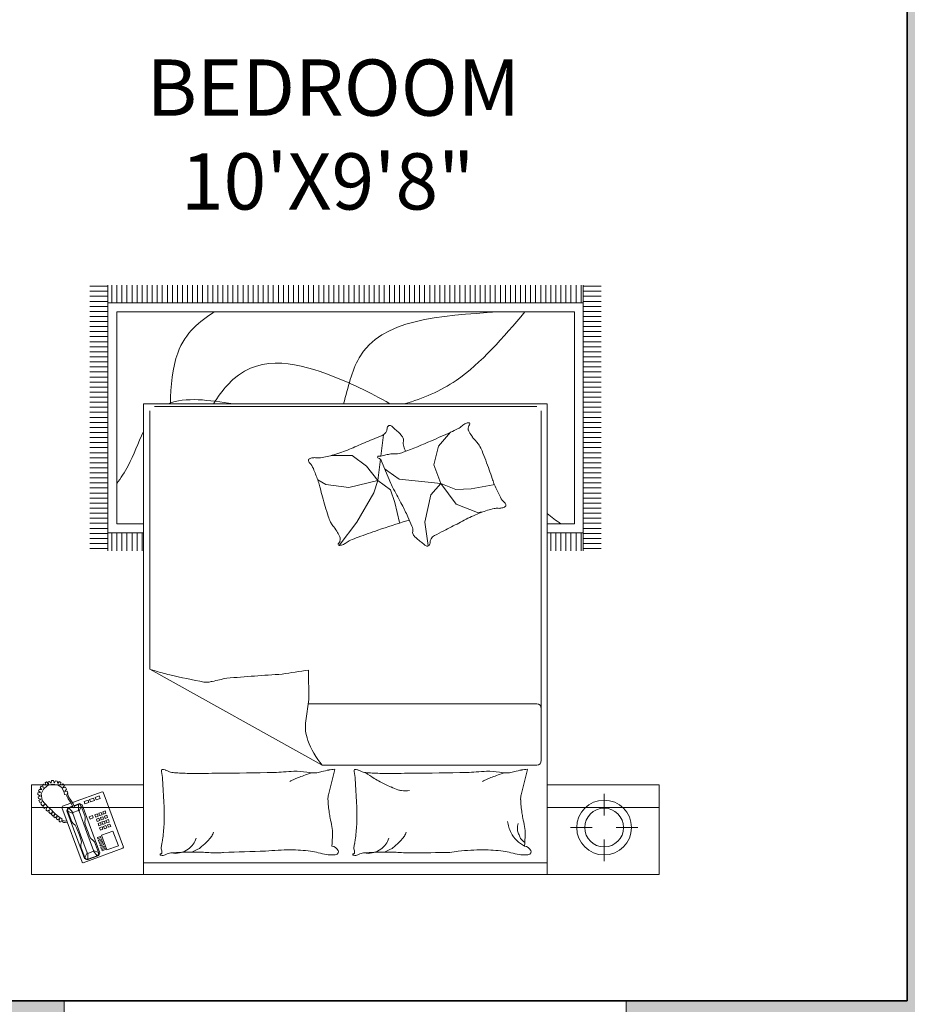
# Model space of a CAD drawing. Units: inches. Extents: x 311 to 815, y -527 to 136.
# Tile 4 of 21: x 445 to 539, y -474 to -368. Entities that reach past the tile are written whole.
import ezdxf

# ---------------------------------------------------------------- set-up
doc = ezdxf.new("R2010")
doc.units = ezdxf.units.IN
doc.header["$MEASUREMENT"] = 0
for name, color, linetype, lineweight in [('A-AREA-IDEN', 8, 'Continuous', 18), ('A-WALL-PATT', 242, 'Continuous', 13), ('wall', 1, 'Continuous', 35), ('win', 5, 'Continuous', 18)]:
    doc.layers.add(name, color=color, linetype=linetype, lineweight=lineweight)
doc.layers.add('furniture', color=50, linetype='Continuous', lineweight=13, transparency=0.8)
doc.styles.add('DIM_FONT', font='SIMPLEX.shx', dxfattribs={"width": 0.8})
doc.styles.get("Standard").update_dxf_attribs({"font": 'arial.ttf'})

# ---------------------------------------------------------------- blocks, each defined once
blk = doc.blocks.new('A$C4F634EDD')
for p, q in [((0, 2.6295), (0, 2.2295)), ((0.5, 2.6295), (0, 2.6295)), ((0.5, 2.6295), (2.3, 2.6295)), ((0.5, 0.5295), (0.5, 2.6295)), ((0.5, 2.2295), (0.5, 2.6295)), ((2.3, 2.6295), (2.3, 0.5295)), ((2.3, 2.6295), (2.8, 2.6295)), ((2.3, 2.2295), (2.3, 2.6295)), ((2.8, 2.6295), (2.8, 2.2295)), ((0.2457, 2.5697), (0.2457, 2.4733)), ((0.5, 2.5771), (2.3, 2.5771)), ((2.392, 2.5115), (2.5692, 2.5765)), ((2.4985, 2.5445), (2.5516, 2.564)), ((2.5062, 2.5454), (2.5487, 2.561)), ((2.5483, 2.5347), (2.5487, 2.561)), ((2.5487, 2.561), (2.5571, 2.56)), ((2.5615, 2.5536), (2.5514, 2.5318)), ((2.5516, 2.564), (2.5637, 2.5584)), ((2.5571, 2.56), (2.5615, 2.5536)), ((2.5615, 2.5536), (2.5791, 2.5058)), ((2.5637, 2.5584), (2.6418, 2.3458)), ((2.5692, 2.5765), (2.574, 2.5743)), ((2.574, 2.5743), (2.6638, 2.3298)), ((2.3898, 2.5066), (2.392, 2.5115)), ((2.4795, 2.2621), (2.3898, 2.5066)), ((2.412, 2.5007), (2.4634, 2.5196)), ((2.4634, 2.5196), (2.4875, 2.454)), ((2.4842, 2.5232), (2.47, 2.518)), ((2.47, 2.518), (2.472, 2.5127)), ((2.472, 2.5127), (2.4862, 2.5179)), ((2.4881, 2.5126), (2.4739, 2.5074)), ((2.4739, 2.5074), (2.4759, 2.502)), ((2.4759, 2.502), (2.4901, 2.5073)), ((2.4862, 2.5179), (2.4842, 2.5232)), ((2.4901, 2.5073), (2.4881, 2.5126)), ((2.4946, 2.5331), (2.4985, 2.5445)), ((2.5734, 2.3187), (2.4946, 2.5331)), ((2.5062, 2.5454), (2.5004, 2.5392)), ((2.5004, 2.5392), (2.5013, 2.5315)), ((2.5013, 2.5315), (2.5188, 2.4836)), ((2.5013, 2.5315), (2.5231, 2.5214)), ((2.5235, 2.5256), (2.5062, 2.5454)), ((2.5231, 2.5214), (2.5235, 2.5256)), ((2.5523, 2.4417), (2.5231, 2.5214)), ((2.5483, 2.5347), (2.5235, 2.5256)), ((2.5514, 2.5318), (2.5483, 2.5347)), ((2.5807, 2.4521), (2.5514, 2.5318)), ((2.5791, 2.5058), (2.5788, 2.4956)), ((2.4361, 2.4352), (2.412, 2.5007)), ((2.492, 2.5019), (2.4778, 2.4967)), ((2.4778, 2.4967), (2.4798, 2.4914)), ((2.4798, 2.4914), (2.494, 2.4966)), ((2.4959, 2.4913), (2.4817, 2.4861)), ((2.4817, 2.4861), (2.4837, 2.4808)), ((2.4837, 2.4808), (2.4979, 2.486)), ((2.4998, 2.4807), (2.4856, 2.4755)), ((2.4856, 2.4755), (2.4876, 2.4702)), ((2.4876, 2.4702), (2.5018, 2.4754)), ((2.5037, 2.47), (2.4895, 2.4648)), ((2.4895, 2.4648), (2.4915, 2.4595)), ((2.4915, 2.4595), (2.5057, 2.4647)), ((2.494, 2.4966), (2.492, 2.5019)), ((2.4979, 2.486), (2.4959, 2.4913)), ((2.5018, 2.4754), (2.4998, 2.4807)), ((2.5057, 2.4647), (2.5037, 2.47)), ((2.5188, 2.4836), (2.5256, 2.4761)), ((2.5256, 2.4761), (2.5342, 2.4692)), ((2.5342, 2.4692), (2.5405, 2.4574)), ((2.5788, 2.4956), (2.5767, 2.4848)), ((2.5767, 2.4848), (2.5795, 2.4717)), ((2.5795, 2.4717), (2.586, 2.454)), ((0.0957, 2.4197), (0.192, 2.4197)), ((0.2994, 2.4197), (0.3957, 2.4197)), ((2.4875, 2.454), (2.4361, 2.4352)), ((2.4457, 2.4146), (2.4563, 2.4185)), ((2.4563, 2.4185), (2.4602, 2.4078)), ((2.4634, 2.4211), (2.474, 2.425)), ((2.4673, 2.4104), (2.4634, 2.4211)), ((2.474, 2.425), (2.4779, 2.4143)), ((2.4811, 2.4276), (2.4917, 2.4315)), ((2.485, 2.4169), (2.4811, 2.4276)), ((2.4956, 2.4208), (2.485, 2.4169)), ((2.4917, 2.4315), (2.4956, 2.4208)), ((2.5405, 2.4574), (2.547, 2.4397)), ((2.5594, 2.4061), (2.547, 2.4397)), ((2.5523, 2.4417), (2.5875, 2.346)), ((2.5807, 2.4521), (2.6158, 2.3564)), ((2.5984, 2.4204), (2.586, 2.454)), ((2.6047, 2.4086), (2.5984, 2.4204)), ((2.4496, 2.4039), (2.4457, 2.4146)), ((2.4602, 2.4078), (2.4496, 2.4039)), ((2.4528, 2.3951), (2.4635, 2.399)), ((2.4567, 2.3844), (2.4528, 2.3951)), ((2.4674, 2.3883), (2.4567, 2.3844)), ((2.46, 2.3756), (2.4706, 2.3795)), ((2.4639, 2.365), (2.46, 2.3756)), ((2.4635, 2.399), (2.4674, 2.3883)), ((2.4779, 2.4143), (2.4673, 2.4104)), ((2.4706, 2.4016), (2.4812, 2.4055)), ((2.4745, 2.3909), (2.4706, 2.4016)), ((2.4706, 2.3795), (2.4745, 2.3689)), ((2.4851, 2.3949), (2.4745, 2.3909)), ((2.4777, 2.3821), (2.4883, 2.386)), ((2.4816, 2.3715), (2.4777, 2.3821)), ((2.4812, 2.4055), (2.4851, 2.3949)), ((2.4922, 2.3754), (2.4816, 2.3715)), ((2.4883, 2.4081), (2.4989, 2.412)), ((2.4922, 2.3975), (2.4883, 2.4081)), ((2.4883, 2.386), (2.4922, 2.3754)), ((2.5028, 2.4014), (2.4922, 2.3975)), ((2.4954, 2.3886), (2.5061, 2.3925)), ((2.4993, 2.378), (2.4954, 2.3886)), ((2.4989, 2.412), (2.5028, 2.4014)), ((2.51, 2.3819), (2.4993, 2.378)), ((2.5026, 2.3691), (2.5132, 2.373)), ((2.5061, 2.3925), (2.51, 2.3819)), ((2.5132, 2.373), (2.5171, 2.3624)), ((2.5238, 2.3769), (2.538, 2.3821)), ((2.5277, 2.3663), (2.5238, 2.3769)), ((2.5419, 2.3715), (2.5277, 2.3663)), ((2.538, 2.3821), (2.5419, 2.3715)), ((2.5622, 2.393), (2.5594, 2.4061)), ((2.5598, 2.372), (2.5601, 2.3822)), ((2.5774, 2.3242), (2.5598, 2.372)), ((2.5601, 2.3822), (2.5622, 2.393)), ((2.6133, 2.4017), (2.6047, 2.4086)), ((2.6201, 2.3941), (2.6133, 2.4017)), ((2.6376, 2.3463), (2.6201, 2.3941)), ((2.6499, 2.3979), (2.6397, 2.3953)), ((2.6417, 2.39), (2.6488, 2.391)), ((2.6488, 2.391), (2.6538, 2.3895)), ((2.6551, 2.397), (2.6499, 2.3979)), ((2.6538, 2.3895), (2.6596, 2.388)), ((2.6627, 2.392), (2.6551, 2.397)), ((2.6596, 2.388), (2.6626, 2.3867)), ((2.6626, 2.3867), (2.6662, 2.388)), ((2.6692, 2.394), (2.6627, 2.392)), ((2.6662, 2.388), (2.6632, 2.3828)), ((2.6632, 2.3828), (2.6736, 2.3744)), ((2.6736, 2.3944), (2.6692, 2.394)), ((2.6765, 2.391), (2.6736, 2.3944)), ((2.6736, 2.3744), (2.6922, 2.3593)), ((2.6742, 2.3795), (2.6765, 2.391)), ((2.6824, 2.3858), (2.6742, 2.3795)), ((2.6873, 2.3815), (2.6824, 2.3858)), ((2.6853, 2.369), (2.6873, 2.3815)), ((2.6946, 2.376), (2.6853, 2.369)), ((2.6995, 2.3713), (2.6946, 2.376)), ((2.695, 2.3603), (2.6995, 2.3713)), ((0, 2.3301), (0.5, 2.3301)), ((0.2457, 2.366), (0.2457, 2.2697)), ((2.8, 2.3301), (2.3, 2.3301)), ((2.4745, 2.3689), (2.4639, 2.365)), ((2.4672, 2.3561), (2.4778, 2.36)), ((2.4711, 2.3455), (2.4672, 2.3561)), ((2.4817, 2.3494), (2.4711, 2.3455)), ((2.4778, 2.36), (2.4817, 2.3494)), ((2.4849, 2.3626), (2.4955, 2.3665)), ((2.4888, 2.352), (2.4849, 2.3626)), ((2.4994, 2.3559), (2.4888, 2.352)), ((2.4955, 2.3665), (2.4994, 2.3559)), ((2.5065, 2.3585), (2.5026, 2.3691)), ((2.5171, 2.3624), (2.5065, 2.3585)), ((2.5774, 2.3242), (2.5875, 2.346)), ((2.5875, 2.346), (2.5905, 2.3431)), ((2.5905, 2.3431), (2.5901, 2.3168)), ((2.6154, 2.3522), (2.5905, 2.3431)), ((2.613, 2.3312), (2.6077, 2.3293)), ((2.6077, 2.3293), (2.6135, 2.3141)), ((2.6192, 2.3174), (2.613, 2.3312)), ((2.6153, 2.3261), (2.6327, 2.3324)), ((2.6158, 2.3564), (2.6154, 2.3522)), ((2.6154, 2.3522), (2.6327, 2.3324)), ((2.6376, 2.3463), (2.6158, 2.3564)), ((2.6369, 2.332), (2.6161, 2.3243)), ((2.6327, 2.3324), (2.6385, 2.3386)), ((2.6418, 2.3458), (2.6369, 2.332)), ((2.6385, 2.3386), (2.6376, 2.3463)), ((2.6638, 2.3298), (2.6616, 2.3249)), ((2.6922, 2.3593), (2.7051, 2.3473)), ((2.7031, 2.3682), (2.695, 2.3603)), ((2.7096, 2.3616), (2.7031, 2.3682)), ((2.7051, 2.3473), (2.7079, 2.3475)), ((2.7062, 2.351), (2.7096, 2.3616)), ((2.7147, 2.3578), (2.7062, 2.351)), ((2.7079, 2.3475), (2.7079, 2.3443)), ((2.7079, 2.3443), (2.727, 2.3277)), ((2.7214, 2.3517), (2.7147, 2.3578)), ((2.7196, 2.34), (2.7214, 2.3517)), ((2.7286, 2.3466), (2.7196, 2.34)), ((2.727, 2.3277), (2.7512, 2.2983)), ((2.7346, 2.3423), (2.7286, 2.3466)), ((2.732, 2.3295), (2.7346, 2.3423)), ((2.7423, 2.3345), (2.732, 2.3295)), ((2.7495, 2.325), (2.7423, 2.3345)), ((2.6172, 2.3086), (2.4844, 2.2599)), ((2.5114, 2.2959), (2.4936, 2.2894)), ((2.4936, 2.2894), (2.4976, 2.2788)), ((2.4976, 2.2788), (2.5153, 2.2853)), ((2.5153, 2.2853), (2.5114, 2.2959)), ((2.5362, 2.305), (2.5185, 2.2985)), ((2.5185, 2.2985), (2.5224, 2.2879)), ((2.5224, 2.2879), (2.5401, 2.2944)), ((2.5401, 2.2944), (2.5362, 2.305)), ((2.561, 2.3141), (2.5433, 2.3076)), ((2.5433, 2.3076), (2.5472, 2.297)), ((2.5472, 2.297), (2.5649, 2.3035)), ((2.5649, 2.3035), (2.561, 2.3141)), ((2.5855, 2.3131), (2.5734, 2.3187)), ((2.5818, 2.3178), (2.5774, 2.3242)), ((2.5901, 2.3168), (2.5818, 2.3178)), ((2.6104, 2.3222), (2.5855, 2.3131)), ((2.5901, 2.3168), (2.6097, 2.324)), ((2.6135, 2.3141), (2.6244, 2.2977)), ((2.626, 2.3069), (2.6192, 2.3174)), ((2.6616, 2.3249), (2.6234, 2.3109)), ((2.6244, 2.2977), (2.6349, 2.2825)), ((2.6365, 2.2916), (2.626, 2.3069)), ((2.6407, 2.2834), (2.6365, 2.2916)), ((2.7406, 2.3172), (2.7495, 2.325)), ((2.7519, 2.3218), (2.7406, 2.3172)), ((2.7512, 2.2983), (2.756, 2.2695)), ((2.7575, 2.3144), (2.7519, 2.3218)), ((2.7526, 2.3045), (2.7575, 2.3144)), ((2.7622, 2.308), (2.7526, 2.3045)), ((2.7574, 2.2924), (2.7673, 2.2997)), ((2.7687, 2.2905), (2.7574, 2.2924)), ((2.7673, 2.2997), (2.7622, 2.308)), ((2.7699, 2.2828), (2.7687, 2.2905)), ((0.5953, 2.1912), (0.616, 2.2738)), ((1.4546, 2.1912), (1.4752, 2.2738)), ((2.4844, 2.2599), (2.4795, 2.2621)), ((2.6349, 2.2825), (2.638, 2.273)), ((2.6399, 2.2712), (2.6374, 2.2659)), ((2.6374, 2.2659), (2.6398, 2.257)), ((2.638, 2.273), (2.6399, 2.2712)), ((2.6398, 2.257), (2.6509, 2.259)), ((2.6438, 2.2739), (2.6407, 2.2834)), ((2.6509, 2.259), (2.6431, 2.2492)), ((2.6431, 2.2492), (2.6473, 2.2398)), ((2.6519, 2.2716), (2.6438, 2.2739)), ((2.6473, 2.2398), (2.6592, 2.2429)), ((2.6535, 2.2628), (2.6519, 2.2716)), ((2.6592, 2.2429), (2.6521, 2.2314)), ((2.6636, 2.2409), (2.6535, 2.2628)), ((2.6836, 2.2287), (2.6636, 2.2409)), ((2.7459, 2.2483), (2.7284, 2.2317)), ((2.756, 2.2695), (2.7459, 2.2483)), ((2.7509, 2.2314), (2.7459, 2.2418)), ((2.7459, 2.2418), (2.7568, 2.2352)), ((2.7529, 2.2505), (2.7645, 2.2498)), ((2.7607, 2.2424), (2.7529, 2.2505)), ((2.7568, 2.2352), (2.7607, 2.2424)), ((2.7587, 2.279), (2.7699, 2.2828)), ((2.7708, 2.2725), (2.7587, 2.279)), ((2.759, 2.2637), (2.7706, 2.2643)), ((2.7676, 2.2559), (2.759, 2.2637)), ((2.7645, 2.2498), (2.7676, 2.2559)), ((2.7706, 2.2643), (2.7708, 2.2725)), ((0, 2.2295), (0.5, 2.2295)), ((2.8, 2.2295), (2.3, 2.2295)), ((2.6521, 2.2314), (2.6598, 2.2248)), ((2.6598, 2.2248), (2.6697, 2.2309)), ((2.6697, 2.2309), (2.6684, 2.219)), ((2.6684, 2.219), (2.6761, 2.2145)), ((2.6761, 2.2145), (2.6821, 2.2237)), ((2.6821, 2.2237), (2.6843, 2.2135)), ((2.7063, 2.2256), (2.6836, 2.2287)), ((2.6843, 2.2135), (2.6927, 2.2117)), ((2.6927, 2.2117), (2.6986, 2.222)), ((2.6986, 2.222), (2.7019, 2.2098)), ((2.7019, 2.2098), (2.7102, 2.2104)), ((2.7284, 2.2317), (2.7063, 2.2256)), ((2.7102, 2.2104), (2.7113, 2.2218)), ((2.7113, 2.2218), (2.7192, 2.2137)), ((2.7192, 2.2137), (2.7255, 2.2152)), ((2.7255, 2.2152), (2.7242, 2.2265)), ((2.7242, 2.2265), (2.7324, 2.2165)), ((2.7324, 2.2165), (2.7386, 2.2208)), ((2.7386, 2.2208), (2.7354, 2.2306)), ((2.7354, 2.2306), (2.7462, 2.2264)), ((2.7462, 2.2264), (2.7509, 2.2314)), ((0.5878, 2.1612), (0.5953, 2.1912)), ((1.4471, 2.1612), (1.4546, 2.1912)), ((0.5258, 2.121), (0.5258, 0.5617)), ((1.5035, 2.141), (0.5458, 2.141)), ((1.5035, 2.141), (2.2716, 1.7136)), ((1.576, 1.9433), (1.5624, 1.8479)), ((0.5458, 1.8684), (1.5653, 1.8684)), ((1.5624, 1.8479), (1.5641, 1.7178)), ((2.2716, 0.5617), (2.2716, 1.7136)), ((0.2586, 1.1753), (0.3386, 1.1753)), ((0.2586, 1.1528), (0.3386, 1.1528)), ((0.3386, 0), (0.3386, 1.1852)), ((0.3486, 1.1052), (0.3486, 1.1852)), ((0.3711, 1.1052), (0.3711, 1.1852)), ((0.3936, 1.1052), (0.3936, 1.1852)), ((0.4161, 1.1052), (0.4161, 1.1852)), ((0.4386, 1.1052), (0.4386, 1.1852)), ((0.4611, 1.1052), (0.4611, 1.1852)), ((0.4836, 1.1052), (0.4836, 1.1852)), ((1.031, 1.1612), (1.0448, 1.0581)), ((1.4276, 1.1611), (1.3484, 1.0571)), ((2.3061, 1.1052), (2.3061, 1.1852)), ((2.3286, 1.1052), (2.3286, 1.1852)), ((2.3511, 1.1052), (2.3511, 1.1852)), ((2.3736, 1.1052), (2.3736, 1.1852)), ((2.3961, 1.1052), (2.3961, 1.1852)), ((2.4186, 1.1052), (2.4186, 1.1852)), ((2.4411, 1.1052), (2.4411, 1.1852)), ((2.4588, 1.1852), (2.4588, 0)), ((2.4588, 1.1753), (2.5388, 1.1753)), ((2.4588, 1.1528), (2.5388, 1.1528)), ((0.2586, 1.1303), (0.3386, 1.1303)), ((0.2586, 1.1078), (0.3386, 1.1078)), ((0.3386, 1.1052), (0.5, 1.1052)), ((2.3, 1.1052), (2.4588, 1.1052)), ((2.4588, 1.1303), (2.5388, 1.1303)), ((2.4588, 1.1078), (2.5388, 1.1078)), ((0.2586, 1.0853), (0.3386, 1.0853)), ((0.2586, 1.0628), (0.3386, 1.0628)), ((0.3786, 1.0652), (0.5, 1.0652)), ((0.3786, 0.12), (0.3786, 1.0652)), ((1.0448, 1.0581), (1.019, 0.936)), ((1.1784, 0.9702), (1.1586, 1.0591)), ((1.3484, 1.0571), (1.2733, 0.9268)), ((2.3, 1.0652), (2.4188, 1.0652)), ((2.4188, 1.0652), (2.4188, 0.12)), ((2.4588, 1.0853), (2.5388, 1.0853)), ((2.4588, 1.0628), (2.5388, 1.0628)), ((0.2586, 1.0403), (0.3386, 1.0403)), ((0.2586, 1.0178), (0.3386, 1.0178)), ((0.8108, 1.0151), (0.7868, 1.0117)), ((0.9054, 0.9773), (0.8108, 1.0151)), ((2.4588, 1.0403), (2.5388, 1.0403)), ((2.4588, 1.0178), (2.5388, 1.0178)), ((0.2586, 0.9953), (0.3386, 0.9953)), ((0.2586, 0.9728), (0.3386, 0.9728)), ((0.9743, 0.8845), (0.9054, 0.9773)), ((1.1982, 0.9129), (1.1784, 0.9702)), ((2.4588, 0.9953), (2.5388, 0.9953)), ((2.4588, 0.9728), (2.5388, 0.9728)), ((0.2586, 0.9503), (0.3386, 0.9503)), ((0.2586, 0.9278), (0.3386, 0.9278)), ((1.019, 0.936), (0.9743, 0.8845)), ((1.2733, 0.9268), (1.2555, 0.8715)), ((2.4588, 0.9503), (2.5388, 0.9503)), ((2.4588, 0.9278), (2.5388, 0.9278)), ((0.2586, 0.9053), (0.3386, 0.9053)), ((0.2586, 0.8828), (0.3386, 0.8828)), ((0.7403, 0.8913), (0.737, 0.8849)), ((0.8384, 0.9085), (0.7403, 0.8913)), ((0.9072, 0.912), (0.8384, 0.9085)), ((0.9743, 0.8845), (0.9072, 0.912)), ((0.9743, 0.8845), (1.0052, 0.802)), ((0.9743, 0.8845), (1.16, 0.8656)), ((1.1973, 0.8853), (1.2203, 0.829)), ((1.2555, 0.8715), (1.1982, 0.9129)), ((1.2555, 0.8715), (1.384, 0.9031)), ((1.384, 0.9031), (1.4868, 0.8892)), ((1.4868, 0.8892), (1.5228, 0.8692)), ((2.4588, 0.9053), (2.5388, 0.9053)), ((2.4588, 0.8828), (2.5388, 0.8828)), ((0.2586, 0.8603), (0.3386, 0.8603)), ((0.2586, 0.8378), (0.3386, 0.8378)), ((1.16, 0.8656), (1.2099, 0.8295)), ((1.2555, 0.8715), (1.2437, 0.7773)), ((1.2555, 0.8715), (1.3049, 0.8082)), ((2.4588, 0.8603), (2.5388, 0.8603)), ((2.4588, 0.8378), (2.5388, 0.8378)), ((0.2586, 0.8153), (0.3386, 0.8153)), ((0.2586, 0.7928), (0.3386, 0.7928)), ((1.0052, 0.802), (0.9846, 0.7194)), ((1.2099, 0.8295), (1.222, 0.8209)), ((1.2203, 0.829), (1.2381, 0.7855)), ((1.3049, 0.8082), (1.3701, 0.7608)), ((2.4588, 0.8153), (2.5388, 0.8153)), ((2.4588, 0.7928), (2.5388, 0.7928)), ((0.2586, 0.7703), (0.3386, 0.7703)), ((0.2586, 0.7478), (0.3386, 0.7478)), ((1.2419, 0.7626), (1.23, 0.668)), ((1.3701, 0.7608), (1.463, 0.7608)), ((2.4588, 0.7703), (2.5388, 0.7703)), ((2.4588, 0.7478), (2.5388, 0.7478)), ((0.2586, 0.7253), (0.3386, 0.7253)), ((0.2586, 0.7028), (0.3386, 0.7028)), ((0.9846, 0.7194), (0.931, 0.6569)), ((2.4588, 0.7253), (2.5388, 0.7253)), ((2.4588, 0.7028), (2.5388, 0.7028)), ((0.2586, 0.6803), (0.3386, 0.6803)), ((2.4588, 0.6803), (2.5388, 0.6803)), ((0.2586, 0.6578), (0.3386, 0.6578)), ((0.2586, 0.6353), (0.3386, 0.6353)), ((2.4588, 0.6578), (2.5388, 0.6578)), ((2.4588, 0.6353), (2.5388, 0.6353)), ((0.2586, 0.6128), (0.3386, 0.6128)), ((0.2586, 0.5903), (0.3386, 0.5903)), ((2.4588, 0.6128), (2.5388, 0.6128)), ((2.4588, 0.5903), (2.5388, 0.5903)), ((0.2586, 0.5678), (0.3386, 0.5678)), ((0.2586, 0.5453), (0.3386, 0.5453)), ((2.3, 0.5295), (0.5, 0.5295)), ((0.5458, 0.5417), (2.2516, 0.5417)), ((2.4588, 0.5678), (2.5388, 0.5678)), ((2.4588, 0.5453), (2.5388, 0.5453)), ((0.2586, 0.5228), (0.3386, 0.5228)), ((0.2586, 0.5003), (0.3386, 0.5003)), ((2.4588, 0.5228), (2.5388, 0.5228)), ((2.4588, 0.5003), (2.5388, 0.5003)), ((0.2586, 0.4778), (0.3386, 0.4778)), ((0.2586, 0.4553), (0.3386, 0.4553)), ((2.4588, 0.4778), (2.5388, 0.4778)), ((2.4588, 0.4553), (2.5388, 0.4553)), ((0.2586, 0.4328), (0.3386, 0.4328)), ((0.2586, 0.4103), (0.3386, 0.4103)), ((2.4588, 0.4328), (2.5388, 0.4328)), ((2.4588, 0.4103), (2.5388, 0.4103)), ((0.2586, 0.3878), (0.3386, 0.3878)), ((0.2586, 0.3653), (0.3386, 0.3653)), ((2.4588, 0.3878), (2.5388, 0.3878)), ((2.4588, 0.3653), (2.5388, 0.3653)), ((0.2586, 0.3428), (0.3386, 0.3428)), ((0.2586, 0.3203), (0.3386, 0.3203)), ((2.4588, 0.3428), (2.5388, 0.3428)), ((2.4588, 0.3203), (2.5388, 0.3203)), ((0.2586, 0.2978), (0.3386, 0.2978)), ((0.2586, 0.2753), (0.3386, 0.2753)), ((2.4588, 0.2978), (2.5388, 0.2978)), ((2.4588, 0.2753), (2.5388, 0.2753)), ((0.2586, 0.2528), (0.3386, 0.2528)), ((0.2586, 0.2303), (0.3386, 0.2303)), ((2.4588, 0.2528), (2.5388, 0.2528)), ((2.4588, 0.2303), (2.5388, 0.2303)), ((0.2586, 0.2078), (0.3386, 0.2078)), ((0.2586, 0.1853), (0.3386, 0.1853)), ((2.4588, 0.2078), (2.5388, 0.2078)), ((2.4588, 0.1853), (2.5388, 0.1853)), ((0.2586, 0.1628), (0.3386, 0.1628)), ((0.2586, 0.1403), (0.3386, 0.1403)), ((2.4588, 0.1628), (2.5388, 0.1628)), ((2.4588, 0.1403), (2.5388, 0.1403)), ((0.2586, 0.1178), (0.3386, 0.1178)), ((0.2586, 0.0953), (0.3386, 0.0953)), ((2.4188, 0.12), (0.3786, 0.12)), ((2.4588, 0.1178), (2.5388, 0.1178)), ((2.4588, 0.0953), (2.5388, 0.0953)), ((0.2586, 0.0728), (0.3386, 0.0728)), ((0.2586, 0.0503), (0.3386, 0.0503)), ((2.4588, 0.08), (0.3386, 0.08)), ((0.3486, 0), (0.3486, 0.08)), ((0.3711, 0), (0.3711, 0.08)), ((0.3936, 0), (0.3936, 0.08)), ((0.4161, 0), (0.4161, 0.08)), ((0.4386, 0), (0.4386, 0.08)), ((0.4611, 0), (0.4611, 0.08)), ((0.4836, 0), (0.4836, 0.08)), ((0.5061, 0), (0.5061, 0.08)), ((0.5286, 0), (0.5286, 0.08)), ((0.5511, 0), (0.5511, 0.08)), ((0.5736, 0), (0.5736, 0.08)), ((0.5961, 0), (0.5961, 0.08)), ((0.6186, 0), (0.6186, 0.08)), ((0.6411, 0), (0.6411, 0.08)), ((0.6636, 0), (0.6636, 0.08)), ((0.6861, 0), (0.6861, 0.08)), ((0.7086, 0), (0.7086, 0.08)), ((0.7311, 0), (0.7311, 0.08)), ((0.7536, 0), (0.7536, 0.08)), ((0.7761, 0), (0.7761, 0.08)), ((0.7986, 0), (0.7986, 0.08)), ((0.8211, 0), (0.8211, 0.08)), ((0.8436, 0), (0.8436, 0.08)), ((0.8661, 0), (0.8661, 0.08)), ((0.8886, 0), (0.8886, 0.08)), ((0.9111, 0), (0.9111, 0.08)), ((0.9336, 0), (0.9336, 0.08)), ((0.9561, 0), (0.9561, 0.08)), ((0.9786, 0), (0.9786, 0.08)), ((1.0011, 0), (1.0011, 0.08)), ((1.0236, 0), (1.0236, 0.08)), ((1.0461, 0), (1.0461, 0.08)), ((1.0686, 0), (1.0686, 0.08)), ((1.0911, 0), (1.0911, 0.08)), ((1.1136, 0), (1.1136, 0.08)), ((1.1361, 0), (1.1361, 0.08)), ((1.1586, 0), (1.1586, 0.08)), ((1.1811, 0), (1.1811, 0.08)), ((1.2036, 0), (1.2036, 0.08)), ((1.2261, 0), (1.2261, 0.08)), ((1.2486, 0), (1.2486, 0.08)), ((1.2711, 0), (1.2711, 0.08)), ((1.2936, 0), (1.2936, 0.08)), ((1.3161, 0), (1.3161, 0.08)), ((1.3386, 0), (1.3386, 0.08)), ((1.3611, 0), (1.3611, 0.08)), ((1.3836, 0), (1.3836, 0.08)), ((1.4061, 0), (1.4061, 0.08)), ((1.4286, 0), (1.4286, 0.08)), ((1.4511, 0), (1.4511, 0.08)), ((1.4736, 0), (1.4736, 0.08)), ((1.4961, 0), (1.4961, 0.08)), ((1.5186, 0), (1.5186, 0.08)), ((1.5411, 0), (1.5411, 0.08)), ((1.5636, 0), (1.5636, 0.08)), ((1.5861, 0), (1.5861, 0.08)), ((1.6086, 0), (1.6086, 0.08)), ((1.6311, 0), (1.6311, 0.08)), ((1.6536, 0), (1.6536, 0.08)), ((1.6761, 0), (1.6761, 0.08)), ((1.6986, 0), (1.6986, 0.08)), ((1.7211, 0), (1.7211, 0.08)), ((1.7436, 0), (1.7436, 0.08)), ((1.7661, 0), (1.7661, 0.08)), ((1.7886, 0), (1.7886, 0.08)), ((1.8111, 0), (1.8111, 0.08)), ((1.8336, 0), (1.8336, 0.08)), ((1.8561, 0), (1.8561, 0.08)), ((1.8786, 0), (1.8786, 0.08)), ((1.9011, 0), (1.9011, 0.08)), ((1.9236, 0), (1.9236, 0.08)), ((1.9461, 0), (1.9461, 0.08)), ((1.9686, 0), (1.9686, 0.08)), ((1.9911, 0), (1.9911, 0.08)), ((2.0136, 0), (2.0136, 0.08)), ((2.0361, 0), (2.0361, 0.08)), ((2.0586, 0), (2.0586, 0.08)), ((2.0811, 0), (2.0811, 0.08)), ((2.1036, 0), (2.1036, 0.08)), ((2.1261, 0), (2.1261, 0.08)), ((2.1486, 0), (2.1486, 0.08)), ((2.1711, 0), (2.1711, 0.08)), ((2.1936, 0), (2.1936, 0.08)), ((2.2161, 0), (2.2161, 0.08)), ((2.2386, 0), (2.2386, 0.08)), ((2.2611, 0), (2.2611, 0.08)), ((2.2836, 0), (2.2836, 0.08)), ((2.3061, 0), (2.3061, 0.08)), ((2.3286, 0), (2.3286, 0.08)), ((2.3511, 0), (2.3511, 0.08)), ((2.3736, 0), (2.3736, 0.08)), ((2.3961, 0), (2.3961, 0.08)), ((2.4186, 0), (2.4186, 0.08)), ((2.4411, 0), (2.4411, 0.08)), ((2.4588, 0.0728), (2.5388, 0.0728)), ((2.4588, 0.0503), (2.5388, 0.0503)), ((0.2586, 0.0278), (0.3386, 0.0278)), ((0.2586, 0.0053), (0.3386, 0.0053)), ((2.4588, 0.0278), (2.5388, 0.0278)), ((2.4588, 0.0053), (2.5388, 0.0053))]:
    blk.add_line(p, q)
for radius in [0.1222, 0.0865]:
    blk.add_circle((0.2457, 2.4197), radius)
for centre, radius, start, end in [((0.5848, 2.5274), 0.0131, 101.2724, 206.5805), ((0.6036, 2.5368), 0.0342, 206.5805, 265.5998), ((0.5999, 2.4516), 0.0904, 90, 101.2724), ((0.5999, 2.3808), 0.1611, 81.5628, 90), ((0.5788, 2.2388), 0.3048, 74.256, 81.5628), ((0.7272, 2.7653), 0.2422, 254.256, 262.4531), ((0.7851, 3.2019), 0.6827, 262.4531, 270), ((0.7851, 3.5682), 1.049, 270, 276.0867), ((0.8402, 3.0514), 0.5293, 276.0867, 280.1899), ((1.1602, -8.1346), 10.6675, 90.30153, 91.21582), ((1.1169, 2.2433), 0.2897, 85.1982, 92.5386), ((1.2142, 3.4021), 0.8732, 265.1982, 269.4243), ((1.4317, 2.2032), 0.3916, 128.3886, 133.8115), ((1.2362, 2.45), 0.0768, 117.2396, 128.3886), ((1.3082, 2.3102), 0.234, 110.8603, 117.2396), ((1.2204, 4.0232), 1.4943, 269.4243, 271.9079), ((1.2995, 2.4357), 0.0992, 126.0864, 143.8234), ((1.2995, 2.4357), 0.0992, 105.9352, 126.0864), ((1.2429, 3.3501), 0.8208, 271.9079, 275.2592), ((1.2995, 2.4357), 0.0992, 85.7841, 105.9352), ((1.3132, 2.5864), 0.0539, 275.2592, 300.6513), ((1.3554, 2.5152), 0.0289, 85.6975, 120.6513), ((1.3556, 2.519), 0.0251, 68.2117, 85.6975), ((1.3739, 2.5288), 0.0156, 158.0096, 201.421), ((1.1177, 2.5413), 0.246, 347.8905, 351.8665), ((1.3634, 2.533), 0.00428, 78.1069, 158.0096), ((1.3288, 2.5111), 0.0328, 351.8665, 21.421), ((1.3647, 2.5395), 0.00232, 258.1069, 19.564), ((1.3637, 2.5391), 0.00342, 19.564, 68.2117), ((1.444, 2.5274), 0.0131, 101.2724, 206.5805), ((1.4628, 2.5368), 0.0342, 206.5805, 265.5998), ((1.4591, 2.4516), 0.0904, 90, 101.2724), ((1.4591, 2.3808), 0.1611, 81.5628, 90), ((1.438, 2.2388), 0.3048, 74.256, 81.5628), ((1.5865, 2.7653), 0.2422, 254.256, 262.4531), ((1.6443, 3.2019), 0.6827, 262.4531, 270), ((1.6443, 3.5682), 1.049, 270, 276.0867), ((1.4785, 15.4878), 12.9656, 271.22425, 272.05324), ((1.97, 2.3805), 0.1524, 92.5386, 100.1899), ((1.9761, 2.2433), 0.2897, 85.1982, 92.5386), ((2.0734, 3.4021), 0.8732, 265.1982, 269.4243), ((2.291, 2.2032), 0.3916, 128.3886, 133.8115), ((2.0954, 2.45), 0.0768, 117.2396, 128.3886), ((2.1674, 2.3102), 0.234, 110.8603, 117.2396), ((2.0797, 4.0232), 1.4943, 269.4243, 271.9079), ((2.1588, 2.4357), 0.0992, 126.0864, 143.8234), ((2.1588, 2.4357), 0.0992, 105.9352, 126.0864), ((2.1021, 3.3501), 0.8208, 271.9079, 275.2592), ((2.1588, 2.4357), 0.0992, 85.7841, 105.9352), ((2.1724, 2.5864), 0.0539, 275.2592, 300.6513), ((2.2146, 2.5152), 0.0289, 85.6975, 120.6513), ((2.2149, 2.519), 0.0251, 68.2117, 85.6975), ((2.2331, 2.5288), 0.0156, 158.0096, 201.421), ((1.977, 2.5413), 0.246, 347.8905, 351.8665), ((2.2226, 2.533), 0.00428, 78.1069, 158.0096), ((2.1881, 2.5111), 0.0328, 351.8665, 21.421), ((2.224, 2.5395), 0.00232, 258.1069, 19.564), ((2.2229, 2.5391), 0.00342, 19.564, 68.2117), ((1.0898, 2.4496), 0.4918, 173.7676, 180), ((0.5462, 2.4142), 0.0899, 41.4429, 53.7359), ((0.5368, 2.3783), 0.1399, 45.0976, 62.7964), ((0.5741, 2.4389), 0.0526, 25.3551, 41.4429), ((0.4851, 2.3967), 0.1511, 21.8149, 25.3551), ((0.5368, 2.3783), 0.1399, 27.3988, 45.0976), ((1.1799, 2.4341), 0.0493, 140.9651, 151.6832), ((1.3165, 2.3233), 0.2252, 133.8115, 140.9651), ((1.2995, 2.4357), 0.0992, 143.8234, 161.5603), ((2.2605, 2.3525), 0.9131, 172.3191, 176.6313), ((1.5522, 2.448), 0.1983, 167.8905, 172.3191), ((1.949, 2.4496), 0.4918, 173.7676, 180), ((2.0391, 2.4341), 0.0493, 140.9651, 151.6832), ((2.1757, 2.3233), 0.2252, 133.8115, 140.9651), ((2.1588, 2.4357), 0.0992, 143.8234, 161.5603), ((3.1198, 2.3525), 0.9131, 172.3191, 176.6313), ((2.4114, 2.448), 0.1983, 167.8905, 172.3191), ((0.8019, 2.4496), 0.204, 180, 189.6844), ((1.4703, 2.5637), 0.882, 189.6844, 192.1984), ((0.4345, 2.3765), 0.2056, 18.7799, 21.8149), ((0.576, 2.4246), 0.0562, 0, 18.7799), ((0.5406, 2.4246), 0.0915, 345.3149, 0), ((0.5368, 2.3783), 0.1399, 16.515, 27.3988), ((0.5368, 2.3783), 0.1399, 5.6311, 16.515), ((1.3127, 2.3625), 0.2002, 151.6832, 156.9972), ((1.6611, 2.4496), 0.204, 180, 189.6844), ((2.3295, 2.5637), 0.882, 189.6844, 192.1984), ((2.1719, 2.3625), 0.2002, 151.6832, 156.9972), ((0.2982, 2.3103), 0.3171, 8.0051, 12.1984), ((2.0266, 2.3663), 0.6787, 176.6313, 181.6331), ((1.1575, 2.3103), 0.3171, 8.0051, 12.1984), ((2.8858, 2.3663), 0.6787, 176.6313, 181.6331), ((-0.0401, 2.2627), 0.6588, 2.6649, 8.0051), ((2.7128, 2.3859), 1.3652, 181.6331, 183.055), ((0.8191, 2.2627), 0.6588, 2.6649, 8.0051), ((3.5721, 2.3859), 1.3652, 181.6331, 183.055), ((0.5503, 2.2902), 0.0677, 345.9548, 2.6649), ((14.9657, 3.0398), 13.6356, 183.05496, 183.50486), ((1.4096, 2.2902), 0.0677, 345.9548, 2.6649), ((15.8249, 3.0398), 13.6356, 183.05496, 183.50486), ((1.1303, 1.9835), 0.2721, 85.9172, 93.5552), ((1.1455, 2.197), 0.058, 69.3257, 85.9172), ((0.9871, 1.7772), 0.5066, 65.6735, 69.3257), ((0.473, 2.8815), 0.7387, 291.6577, 293.4844), ((0.473, 2.8815), 0.7387, 293.4844, 295.3111), ((0.6058, 0.9338), 1.4323, 63.5015, 65.6735), ((1.1054, 1.9358), 0.3126, 57.865, 63.5015), ((0.8841, 1.5835), 0.7286, 54.1737, 57.865), ((1.6762, 2.2258), 0.3212, 183.5049, 189.9984), ((1.3322, 2.8815), 0.7387, 291.6577, 293.4844), ((1.3322, 2.8815), 0.7387, 293.4844, 295.3111), ((2.5355, 2.2258), 0.3212, 183.5049, 189.9984), ((0.5887, 2.1609), 0.000917, 165.9551, 274.0829), ((0.5695, 2.4301), 0.2708, 274.0829, 279.4841), ((0.5763, 2.3896), 0.2297, 279.4841, 287.3864), ((0.6807, 2.0561), 0.1197, 96.4341, 107.3864), ((0.6836, 2.0301), 0.1459, 78.4414, 96.4341), ((0.473, 2.8815), 0.7387, 287.1982, 289.428), ((0.759, 2.3985), 0.2301, 258.4414, 272.7491), ((0.473, 2.8815), 0.7387, 289.428, 291.6577), ((0.7026, 3.5718), 1.4048, 272.7491, 274.6176), ((0.9136, 0.9591), 1.2165, 92.6096, 94.6176), ((1.2501, -19.8405), 22.0183, 90.37908, 91.01965), ((1.2012, -3.5404), 5.7185, 89.7135, 90.9704), ((1.224, 1.0141), 1.164, 86.426, 89.7135), ((1.2875, 2.0302), 0.1459, 77.131, 86.426), ((1.3099, 2.1283), 0.0453, 62.7159, 77.131), ((1.3658, 2.2367), 0.0767, 242.7159, 253.7788), ((1.3688, 2.247), 0.0875, 253.7788, 262.8796), ((1.3581, 2.1615), 0.00132, 262.8796, 343.3022), ((1.3409, 2.1667), 0.0193, 343.3022, 9.9984), ((1.448, 2.1609), 0.000917, 165.9551, 274.0829), ((1.4288, 2.4301), 0.2708, 274.0829, 279.4841), ((1.4355, 2.3896), 0.2297, 279.4841, 287.3864), ((1.5399, 2.0561), 0.1197, 96.4341, 107.3864), ((1.5429, 2.0301), 0.1459, 78.4414, 96.4341), ((1.3322, 2.8815), 0.7387, 287.1982, 289.428), ((1.6182, 2.3985), 0.2301, 258.4414, 272.7491), ((1.3322, 2.8815), 0.7387, 289.428, 291.6577), ((1.5619, 3.5718), 1.4048, 272.7491, 274.6176), ((1.7729, 0.9591), 1.2165, 92.6096, 94.6176), ((2.1093, -19.8405), 22.0183, 90.37908, 91.01965), ((2.0605, -3.5404), 5.7185, 89.7135, 90.9704), ((2.0833, 1.0141), 1.164, 86.426, 89.7135), ((2.1467, 2.0302), 0.1459, 77.131, 86.426), ((2.1691, 2.1283), 0.0453, 62.7159, 77.131), ((2.2251, 2.2367), 0.0767, 242.7159, 253.7788), ((2.2281, 2.247), 0.0875, 253.7788, 262.8796), ((2.2174, 2.1615), 0.00132, 262.8796, 343.3022), ((2.2001, 2.1667), 0.0193, 343.3022, 9.9984), ((0.5458, 2.121), 0.02, 90, 180), ((1.2147, 1.9017), 0.3751, 20.1488, 39.6445), ((1.3977, 1.9688), 0.1801, 351.8644, 20.1488), ((0.5458, 1.8884), 0.02, 180, 270), ((1.4194, 4.2174), 2.5158, 281.6741, 283.1904), ((2.0378, 1.5789), 0.1942, 97.7304, 103.1904), ((2.0195, 1.7137), 0.0581, 79.2724, 97.7304), ((1.2737, -2.2227), 4.0646, 77.0745, 79.2724), ((1.0582, 5.4638), 3.7801, 277.692, 279.495), ((0.6102, 18.0525), 16.3521, 273.75703, 274.62393), ((2.0359, 1.0981), 0.6574, 74.0648, 77.0745), ((1.7125, -0.0344), 1.8351, 72.2636, 74.0648), ((0.9863, 1.1494), 0.0359, 297.2902, 3.2455), ((1.0348, 1.1521), 0.0127, 51.1864, 183.2455), ((0.9991, 1.1077), 0.0697, 45.8726, 51.1864), ((1.0791, 1.1902), 0.0452, 225.8726, 232.4713), ((1.2846, 1.4577), 0.3825, 232.4713, 233.7837), ((0.6683, 0.6162), 0.6605, 52.7849, 53.7837), ((0.9362, 0.9689), 0.2176, 46.4776, 52.7849), ((1.3469, 1.2115), 0.0792, 292.7069, 308.5854), ((1.4338, 1.1026), 0.0601, 110.3452, 128.5854), ((1.4251, 1.1259), 0.0352, 86.0516, 110.3452), ((1.4996, 1.1284), 0.0771, 169.5926, 177.2714), ((1.4376, 1.1398), 0.0142, 126.5792, 169.5926), ((1.4273, 1.1567), 0.00443, 13.2808, 86.0516), ((1.4254, 1.1562), 0.0063, 306.5792, 13.2808), ((-0.4173, 3.8699), 3.0972, 296.4147, 297.2902), ((1.0327, 1.0706), 0.0774, 35.8936, 46.4776), ((1.0771, 1.1027), 0.0226, 351.9508, 35.8936), ((1.1449, 1.0931), 0.0458, 171.9508, 202.4162), ((-0.4107, 5.9078), 5.0942, 289.0836, 290.1287), ((1.0543, 1.9106), 0.8371, 290.1287, 292.7069), ((1.4378, 1.1314), 0.0153, 177.2714, 194.5709), ((1.4611, 1.1374), 0.0393, 194.5709, 206.8179), ((1.7401, 1.2785), 0.352, 206.8179, 210.9056), ((-1.8336, 6.2238), 5.8383, 297.49208, 297.84822), ((3.744, -4.3336), 6.1019, 117.49986, 117.84822), ((1.8575, -0.7096), 2.0162, 116.4147, 117.4999), ((2.032, 1.4591), 1.0054, 202.4162, 205.0529), ((0.2266, 4.0657), 3.145, 286.6085, 289.0836), ((1.6045, 1.1973), 0.194, 210.9056, 219.7005), ((1.3929, 1.0217), 0.081, 26.0735, 39.7005), ((1.2892, 0.9709), 0.1965, 17.8396, 26.0735), ((0.6422, 1.4168), 0.43, 282.6252, 290.7486), ((0.5736, 1.5979), 0.6236, 290.7486, 297.4921), ((1.0922, 1.1636), 0.1166, 280.7366, 286.6085), ((2.6493, 1.7476), 1.6868, 205.0529, 207.0884), ((-0.4304, 0.4175), 2.003, 15.2625, 17.8396), ((0.6894, 0.9832), 0.0058, 121.6917, 179.0386), ((0.7004, 0.983), 0.0168, 179.0386, 229.4914), ((0.7131, 0.9448), 0.0509, 103.0402, 121.6917), ((0.6405, 0.9128), 0.0755, 26.3332, 49.4914), ((0.7152, 0.9361), 0.0599, 86.6119, 103.0402), ((0.7224, 1.0587), 0.063, 266.6119, 282.6252), ((2.541, 1.6922), 1.5652, 207.0884, 209.936), ((-1.6775, -0.2344), 2.6619, 25.1732, 26.3332), ((-0.0881, 0.5109), 1.6481, 13.841, 15.2625), ((0.5689, 0.8213), 0.1798, 20.7081, 25.1732), ((0.2268, 0.692), 0.5454, 18.2369, 20.7081), ((0.9989, 0.8042), 0.2143, 22.2355, 29.936), ((2.0418, 1.0357), 0.5454, 193.841, 196.3122), ((1.6908, 0.933), 0.1798, 196.3122, 200.7773), ((2.3102, 1.3785), 1.6481, 198.2369, 199.6584), ((4.0115, 1.8135), 2.6619, 200.7773, 201.9373), ((2.6444, 1.4979), 2.003, 199.6584, 202.2355), ((1.6124, 0.8472), 0.0755, 201.9373, 225.0955), ((1.5473, 0.7819), 0.0168, 354.6428, 45.0955), ((1.1834, 0.6373), 0.1166, 98.1216, 111.0043), ((1.1763, 0.687), 0.0663, 85.4882, 98.1216), ((1.1871, 0.8241), 0.0712, 265.4882, 277.6784), ((1.1727, 0.9313), 0.1794, 277.6784, 284.8807), ((1.2689, 0.569), 0.1955, 97.9822, 104.8807), ((1.2594, 0.7942), 0.0231, 202.2355, 252.8133), ((1.2465, 0.729), 0.034, 85.7407, 97.9822), ((1.2497, 0.772), 0.0092, 265.7407, 289.3799), ((1.2512, 0.7678), 0.00467, 289.3799, 72.8133), ((1.6266, 0.159), 0.6236, 106.3527, 113.0962), ((1.5721, 0.3449), 0.43, 98.2293, 106.3527), ((1.5195, 0.708), 0.063, 82.216, 98.2293), ((1.5362, 0.8298), 0.0599, 262.216, 278.6443), ((1.5375, 0.8209), 0.0509, 278.6443, 297.2959), ((1.5582, 0.7808), 0.0058, 297.2959, 354.6428), ((0.9722, 0.8143), 0.1965, 202.2355, 210.4694), ((0.8727, 0.7557), 0.081, 210.4694, 224.0964), ((2.2689, -2.1899), 3.145, 111.0043, 113.4795), ((0.1831, 0.4093), 1.0054, 18.0203, 19.3448), ((1.0957, 0.7061), 0.0458, 347.5549, 18.0203), ((0.5234, 2.5582), 2.0162, 292.0188, 293.104), ((-1.0798, 6.3161), 6.1019, 293.10398, 293.45234), ((3.6722, -4.6377), 5.8383, 113.0962, 113.45234), ((0.6752, 0.5644), 0.194, 35.3015, 44.0964), ((0.5462, 0.4731), 0.352, 31.2138, 35.3015), ((3.0455, -3.9778), 5.0942, 113.4795, 114.5246), ((1.1625, 0.6914), 0.0226, 167.5549, 211.4977), ((1.2092, 0.72), 0.0774, 211.4977, 222.0817), ((1.3133, 0.814), 0.2176, 222.0817, 228.389), ((1.2495, 0.6379), 0.0359, 112.8944, 178.8496), ((2.4404, -2.1823), 3.0972, 112.0188, 112.8944), ((0.8506, 0.6191), 0.0063, 130.9751, 197.6767), ((0.8488, 0.6185), 0.00443, 197.6767, 270.4475), ((0.8372, 0.6345), 0.0142, 310.9751, 353.9885), ((0.8136, 0.6351), 0.0393, 18.9668, 31.2138), ((0.8486, 0.6493), 0.0352, 270.4475, 294.7411), ((0.8364, 0.6429), 0.0153, 1.6673, 18.9668), ((0.7746, 0.6411), 0.0771, 353.9885, 1.6673), ((0.8382, 0.6719), 0.0601, 294.7411, 312.9813), ((0.9332, 0.57), 0.0792, 117.1028, 132.9813), ((1.2784, -0.1047), 0.8371, 114.5246, 117.1028), ((1.6074, 1.1451), 0.6605, 228.389, 229.3878), ((0.9284, 0.3533), 0.3825, 48.0754, 49.3878), ((1.1538, 0.6043), 0.0452, 41.4767, 48.0754), ((1.2399, 0.6804), 0.0697, 221.4767, 226.7905), ((1.2009, 0.6389), 0.0127, 226.7905, 358.8496)]:
    blk.add_arc(centre, radius, start, end)
for points in [[(0.4393, 1.0652), (0.4595, 1.05), (0.4798, 1.0348), (0.5, 1.0195)], [(1.9003, 0.5295), (2.0065, 0.514), (2.1132, 0.4978), (2.1894, 0.5295)]]:
    blk.add_open_spline(points, degree=3)
for points, knots in [([(2.3, 0.6535), (2.3236, 0.7026), (2.3554, 0.7914), (2.4015, 0.8608), (2.4188, 0.8868)], [1893.525221, 1893.525221, 1893.525221, 1893.525221, 2051.902476, 2146.74457, 2146.74457, 2146.74457, 2146.74457]), ([(0.5992, 0.12), (0.6957, 0.2341), (0.8523, 0.4189), (1.0536, 0.5069), (1.136, 0.5295)], [0, 0, 0, 0, 432.822832, 701.445452, 701.445452, 701.445452, 701.445452]), ([(0.7187, 0.12), (0.9791, 0.1362), (1.326, 0.1577), (1.3868, 0.4574), (1.408, 0.5295)], [0, 0, 0, 0, 653.160442, 870.050857, 870.050857, 870.050857, 870.050857]), ([(1.2016, 0.5295), (1.2892, 0.479), (1.5144, 0.3684), (1.8265, 0.2994), (1.9681, 0.4992), (1.9875, 0.5295)], [936.534237, 936.534237, 936.534237, 936.534237, 1243.285375, 1683.261222, 1758.254386, 1758.254386, 1758.254386, 1758.254386]), ([(2.1796, 0.5295), (2.1798, 0.4519), (2.1548, 0.2369), (2.0487, 0.164), (1.9846, 0.12)], [2202.034493, 2202.034493, 2202.034493, 2202.034493, 2357.807635, 2594.446174, 2594.446174, 2594.446174, 2594.446174])]:
    blk.add_open_spline(points, degree=3, knots=knots)
at = {"style": 'DIM_FONT', "width": 0.8, "flags": 9}
for tag, p in [('YSIZE', (0.5, 2.6295)), ('XSIZE', (0.5, 2.6295)), ('XSIZE', (2.2985, 2.6295)), ('YSIZE', (2.2985, 2.6295))]:
    blk.add_attdef(tag, p, '', height=0.0005, dxfattribs=at)
blk = doc.blocks.new('WIN-60IN')
for p, q in [((9, 60), (0, 60)), ((3.5, 0), (3.5, 60)), ((5.5, 0), (5.5, 60)), ((9, 0), (0, 0))]:
    blk.add_line(p, q)

msp = doc.modelspace()

# ---------------------------------------------------------------- hatches: boundary and pattern name
at = {"layer": 'A-WALL-PATT'}
h = msp.add_hatch(color=256, dxfattribs=at)
h.dxf.hatch_style = 1
h.paths.add_polyline_path([(557.82, 21.87), (509.32, 21.87), (509.32, 12.87), (539.32, 12.87), (539.32, -112.13), (548.32, -112.13), (548.32, -58.63), (557.82, -58.63), (557.82, -49.63), (548.32, -49.63), (548.32, 12.87), (557.82, 12.87)])
h.paths.add_polyline_path([(449.32, 21.87), (410.32, 21.87), (410.32, -15.13), (419.32, -15.13), (419.32, 12.87), (449.32, 12.87)])
h.paths.add_polyline_path([(626.82, 21.87), (581.82, 21.87), (581.82, 12.87), (591.32, 12.87), (591.32, -49.63), (581.82, -49.63), (581.82, -58.63), (591.32, -58.63), (591.32, -112.13), (600.32, -112.13), (600.32, 12.87), (626.82, 12.87)])
h.paths.add_polyline_path([(722.32, 21.87), (686.82, 21.87), (686.82, 12.87), (713.32, 12.87), (713.32, -18.13), (722.32, -18.13)])
h.paths.add_polyline_path([(722.32, -42.13), (713.32, -42.13), (713.32, -73.13), (722.32, -73.13)])
h.paths.add_polyline_path([(501.32, -103.13), (419.32, -103.13), (419.32, -75.13), (410.32, -75.13), (410.32, -126.63), (419.32, -126.63), (419.32, -112.13), (492.32, -112.13), (492.32, -143.13), (501.32, -143.13)])
h.paths.add_polyline_path([(548.32, -165.13), (419.32, -165.13), (419.32, -150.63), (410.32, -150.63), (410.32, -202.13), (419.32, -202.13), (419.32, -174.13), (548.32, -174.13)])
h.paths.add_polyline_path([(722.32, -103.13), (636.32, -103.13), (636.32, -112.13), (713.32, -112.13), (713.32, -140.13), (722.32, -140.13)])
h.paths.add_polyline_path([(548.32, -210.13), (539.32, -210.13), (539.32, -290.13), (419.32, -290.13), (419.32, -262.13), (410.32, -262.13), (410.32, -311.57), (419.32, -311.57), (419.32, -299.13), (469.32, -299.13), (469.32, -348.13), (443.32, -348.13), (443.32, -357.13), (478.32, -357.13), (478.32, -299.13), (548.32, -299.13)])
h.paths.add_polyline_path([(722.32, -200.13), (713.32, -200.13), (713.32, -228.13), (609.32, -228.13), (609.32, -237.13), (713.32, -237.13), (713.32, -262.63), (722.32, -262.63)])
h.paths.add_polyline_path([(722.32, -322.63), (713.32, -322.63), (713.32, -348.13), (633.32, -348.13), (633.32, -357.13), (713.32, -357.13), (713.32, -385.13), (722.32, -385.13)])
h.paths.add_polyline_path([(419.32, -335.57), (410.32, -335.57), (410.32, -390.84), (419.32, -390.84)])
h.paths.add_polyline_path([(419.32, -450.84), (410.32, -450.84), (410.32, -482.13), (449.32, -482.13), (449.32, -473.13), (419.32, -473.13)])
h.paths.add_polyline_path([(582.82, -473.13), (548.32, -473.13), (548.32, -348.13), (539.32, -348.13), (539.32, -473.13), (509.32, -473.13), (509.32, -482.13), (582.82, -482.13)])
h.paths.add_polyline_path([(722.32, -445.13), (713.32, -445.13), (713.32, -473.13), (678.82, -473.13), (678.82, -482.13), (722.32, -482.13)])

# ---------------------------------------------------------------- linework, layer by layer
at = {"layer": 'wall'}
for p, q in [((539.32, -473.13), (539.32, -348.13)), ((419.32, -473.13), (539.32, -473.13))]:
    msp.add_line(p, q, dxfattribs=at)

# ---------------------------------------------------------------- block references
at = {"layer": 'furniture', "xscale": 23.93855799564961, "yscale": 23.93855799564961, "zscale": 23.93855799564961, "rotation": 180}
msp.add_blockref('A$C4F634EDD', (512.84, -396.72), dxfattribs=at)
at = {"layer": 'win', "rotation": 90.00000000000003}
msp.add_blockref('WIN-60IN', (509.32, -482.13), dxfattribs=at)

# ---------------------------------------------------------------- texts
at = {"layer": 'A-AREA-IDEN', "insert": (450.77, -372.64), "char_height": 6.0073, "attachment_point": 1}
msp.add_mtext_dynamic_manual_height_columns('    BEDROOM\\P      10\'X9\'8"', width=59.0599, gutter_width=1, heights=[0], dxfattribs=at)

doc.saveas('drawing.dxf')
